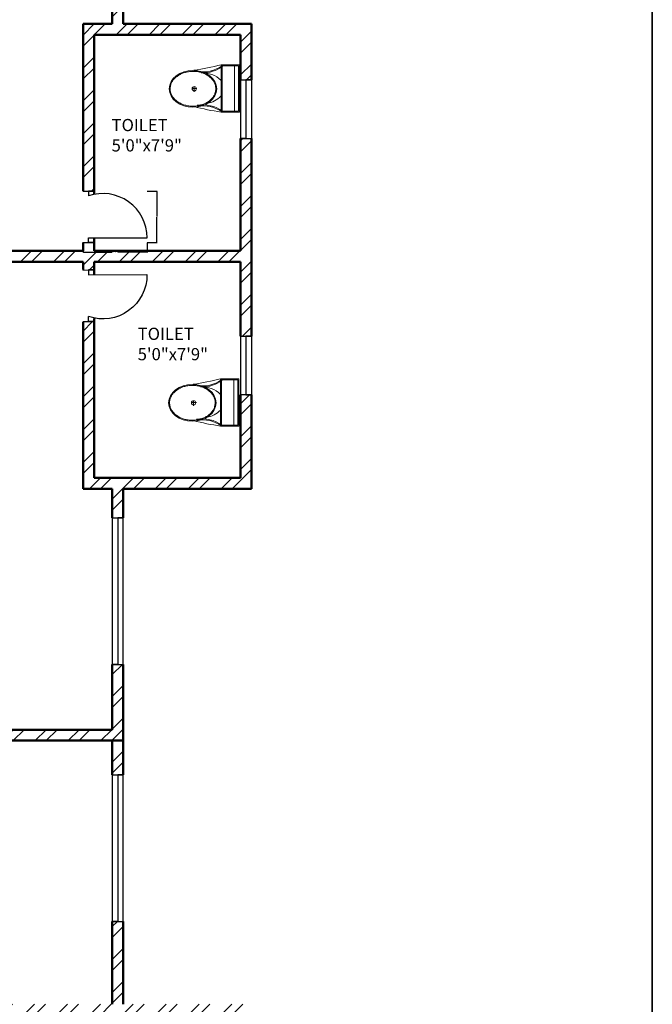
# Model space of a CAD drawing. Units: inches. Extents: x 963 to 2075, y 289 to 2657.
# Tile 58 of 98: x 1815 to 2075, y 1714 to 2117. Entities that reach past the tile are written whole.
import ezdxf

# ---------------------------------------------------------------- set-up
doc = ezdxf.new("R2010")
doc.units = ezdxf.units.IN
for name, color, linetype, lineweight in [('A-ANNO-DIMS', 2, 'Continuous', 18), ('A-ANNO-TTLB', 7, 'Continuous', 35), ('A-AREA-IDEN', 7, 'Continuous', 18), ('A-DOOR', 4, 'Continuous', 25), ('A-FLOR-FIXT', 9, 'Continuous', 18), ('A-GLAZ', 3, 'Continuous', 25), ('A-WALL', 7, 'Continuous', 50), ('A-WALL-PATT', 8, 'Continuous', 13)]:
    doc.layers.add(name, color=color, linetype=linetype, lineweight=lineweight)
doc.styles.get("Standard").update_dxf_attribs({"font": 'arial.ttf'})
doc.dimstyles.get("Standard").update_dxf_attribs({"dimtxt": 0.18, "dimasz": 0.18, "dimexe": 0.18, "dimexo": 0.0625, "dimgap": 0.09, "dimtad": 0, "dimtih": 1, "dimtoh": 1, "dimdec": 4, "dimzin": 0, "dimdsep": 46, "dimtxsty": 'Standard', "dimcen": 0.09, "dimadec": 0, "dimazin": 0, "dimtfac": 1, "dimtdec": 4, "dimtofl": 0, "dimtmove": 0, "dimatfit": 3, "dimfxl": 1, "dimtolj": 1, "dimtzin": 0, "dimarcsym": 0})

# ---------------------------------------------------------------- blocks, each defined once
blk = doc.blocks.new('A$C31115884')
for p, q in [((283, 498), (223, 498)), ((258, 466), (258, 523)), ((0, 200), (0, 0)), ((520, 200), (0, 200)), ((10, 190), (10, 10)), ((510, 190), (10, 190)), ((510, 10), (510, 190)), ((520, 0), (520, 200)), ((510, 54), (0, 54)), ((10, 10), (510, 10)), ((0, 0), (520, 0))]:
    blk.add_line(p, q)
blk.add_circle((256, 496), 23.6)
for centre, radius, start, end in [((2778, -205), 2807, 165.4549, 171.7133), ((-295, 403), 365, 324.2091, 9.3499), ((-295, 403), 375, 324.2091, 9.3499), ((806, 403), 365, 170.6501, 215.7909), ((3237, 905), 2807, 188.2867, 194.5451), ((384, 406), 293, 190.2774, 224.1564), ((139, 406), 293, 315.8436, 2.6563), ((806, 403), 375, 179.2036, 215.7909)]:
    blk.add_arc(centre, radius, start, end)
blk.add_ellipse((256, 510), major_axis=(0, -261), ratio=0.772727)
blk.add_open_spline([(256, 259), (263, 259), (270, 260), (288, 262), (299, 265), (320, 273), (330, 278), (350, 291), (360, 299), (378, 316), (386, 326), (402, 347), (409, 358), (421, 383), (427, 395), (436, 422), (440, 436), (445, 465), (447, 480), (448, 509), (448, 524), (445, 553), (443, 568), (436, 596), (432, 610), (422, 636), (416, 649), (402, 672), (395, 683), (379, 703), (370, 712), (351, 728), (341, 735), (321, 746), (310, 751), (289, 757), (278, 759), (256, 761), (245, 761), (223, 757), (212, 754), (191, 746), (181, 741), (161, 728), (151, 720), (133, 703), (125, 693), (110, 672), (103, 660), (90, 636), (85, 623), (76, 596), (72, 582), (67, 553), (66, 538), (64, 509), (65, 494), (68, 465), (70, 450), (77, 422), (81, 408), (91, 382), (97, 370), (111, 346), (118, 335), (135, 316), (144, 307), (162, 291), (172, 284), (193, 273), (203, 269), (225, 262), (236, 260), (250, 259), (253, 259), (256, 259)], degree=3, knots=[0, 0, 0, 0, 0.110105, 0.110105, 0.285049, 0.285049, 0.459994, 0.459994, 0.634938, 0.634938, 0.809882, 0.809882, 0.984827, 0.984827, 1.159771, 1.159771, 1.334715, 1.334715, 1.50966, 1.50966, 1.684604, 1.684604, 1.859549, 1.859549, 2.034493, 2.034493, 2.209437, 2.209437, 2.384382, 2.384382, 2.559326, 2.559326, 2.73427, 2.73427, 2.909215, 2.909215, 3.084159, 3.084159, 3.259103, 3.259103, 3.434048, 3.434048, 3.608992, 3.608992, 3.783936, 3.783936, 3.958881, 3.958881, 4.133825, 4.133825, 4.30877, 4.30877, 4.483714, 4.483714, 4.658658, 4.658658, 4.833603, 4.833603, 5.008547, 5.008547, 5.183491, 5.183491, 5.358436, 5.358436, 5.53338, 5.53338, 5.708324, 5.708324, 5.883269, 5.883269, 6.058213, 6.058213, 6.233158, 6.233158, 6.283185, 6.283185, 6.283185, 6.283185])
blk = doc.blocks.new('DOOR-2')
for p, q in [((0, 21.1), (4.5, 21.1)), ((4.5, 21.1), (2.25, 21.1)), ((2.25, 21.1), (2.25, 19.1)), ((0, 0), (4.5, 0)), ((2.25, 0), (2.25, 2)), ((2.25, 2), (26.25, 2)), ((4.5, 0), (2.25, 0))]:
    blk.add_line(p, q)
blk.add_arc((8.16, 2), 18.09, 0, 109.0656)
blk = doc.blocks.new('*D32')
at = {"layer": 'A-ANNO-DIMS', "color": 0, "lineweight": -2, "transparency": 16777216}
for p, q in [((1841.42, 2025.79), (1841.42, 2021.73)), ((1867.67, 2025.79), (1867.67, 2021.73)), ((1841.6, 2021.91), (1853.42, 2021.91)), ((1867.49, 2021.91), (1855.68, 2021.91))]:
    blk.add_line(p, q, dxfattribs=at)
at = {"layer": 'A-ANNO-DIMS', "color": 0, "transparency": 16777216}
for points in [[(1841.6, 2021.94), (1841.6, 2021.88), (1841.42, 2021.91)], [(1867.49, 2021.94), (1867.49, 2021.88), (1867.67, 2021.91)]]:
    blk.add_solid(points, dxfattribs=at)
at = {"layer": 'Defpoints', "color": 0, "transparency": 16777216}
for p in [(1841.42, 2025.85), (1867.67, 2025.85), (1867.67, 2021.91)]:
    blk.add_point(p, dxfattribs=at)
at = {"layer": 'A-ANNO-DIMS', "color": 0, "transparency": 16777216, "insert": (1854.55, 2021.91), "char_height": 0.18, "attachment_point": 5}
blk.add_mtext('\\A1;DOOR D2 26 TYP.', dxfattribs=at)
blk = doc.blocks.new('*D33')
at = {"layer": 'A-ANNO-DIMS', "color": 0, "lineweight": -2, "transparency": 16777216}
for p, q in [((1867.73, 2046.95), (1871.79, 2046.95)), ((1871.61, 2046.77), (1871.61, 2036.58)), ((1871.61, 2026.03), (1871.61, 2036.22)), ((1867.73, 2025.85), (1871.79, 2025.85))]:
    blk.add_line(p, q, dxfattribs=at)
at = {"layer": 'A-ANNO-DIMS', "color": 0, "transparency": 16777216}
for points in [[(1871.58, 2046.77), (1871.64, 2046.77), (1871.61, 2046.95)], [(1871.58, 2026.03), (1871.64, 2026.03), (1871.61, 2025.85)]]:
    blk.add_solid(points, dxfattribs=at)
at = {"layer": 'Defpoints', "color": 0, "transparency": 16777216}
for p in [(1867.67, 2046.95), (1871.61, 2046.95), (1867.67, 2025.85)]:
    blk.add_point(p, dxfattribs=at)
at = {"layer": 'A-ANNO-DIMS', "color": 0, "transparency": 16777216, "insert": (1871.61, 2036.4), "char_height": 0.18, "attachment_point": 5}
blk.add_mtext('\\A1;21 TYP.', dxfattribs=at)

msp = doc.modelspace()

# ---------------------------------------------------------------- hatches: boundary and pattern name
at = {"layer": 'A-WALL-PATT'}
h = msp.add_hatch(dxfattribs=at)
h.set_pattern_fill('ANSI32', color=256)
h.paths.add_polyline_path([(1296.92, 2558.32), (1203.92, 2558.32), (1203.92, 2493.82), (1191.53, 2493.82), (1191.53, 2489.32), (1211.06, 2489.32), (1211.06, 2492.02), (1211.06, 2493.82), (1208.42, 2493.82), (1208.42, 2553.82), (1292.42, 2553.82), (1292.42, 2538.86), (1296.92, 2538.86)])
h.paths.add_polyline_path([(1442.42, 2558.32), (1349.42, 2558.32), (1349.42, 2538.94), (1353.92, 2538.94), (1353.92, 2553.82), (1437.92, 2553.82), (1437.92, 2493.82), (1434.54, 2493.82), (1434.54, 2489.32), (1448.31, 2489.32), (1448.31, 2491.57), (1448.31, 2493.82), (1442.42, 2493.82)])
h.paths.add_polyline_path([(1415.55, 2491.57), (1415.55, 2493.82), (1340.94, 2493.82), (1340.94, 2489.32), (1371.92, 2489.32), (1371.92, 2378.32), (1367.6, 2378.32), (1367.6, 2373.82), (1371.92, 2373.82), (1371.92, 2355.19), (1376.42, 2355.19), (1376.42, 2489.32), (1415.55, 2489.32)])
h.paths.add_polyline_path([(1304.94, 2491.57), (1304.94, 2493.82), (1296.92, 2493.82), (1296.92, 2514.86), (1292.42, 2514.86), (1292.42, 2493.82), (1232.81, 2493.82), (1232.81, 2489.32), (1256.42, 2489.32), (1256.42, 2327.32), (1253.71, 2327.32), (1253.71, 2322.82), (1328.42, 2322.82), (1328.42, 2331.15), (1323.92, 2331.15), (1323.92, 2327.32), (1260.92, 2327.32), (1260.92, 2373.82), (1323.92, 2373.82), (1323.92, 2357.81), (1328.42, 2357.81), (1328.42, 2373.82), (1346.01, 2373.82), (1346.01, 2376.07), (1346.01, 2378.32), (1260.92, 2378.32), (1260.92, 2489.32), (1304.94, 2489.32)])
h.paths.add_polyline_path([(1226.65, 2327.32), (1124.42, 2327.32), (1124.42, 2347.45), (1119.92, 2347.45), (1119.92, 2322.82), (1163.42, 2322.82), (1163.42, 2305.43), (1165.67, 2305.43), (1167.92, 2305.43), (1167.92, 2322.82), (1226.65, 2322.82), (1226.65, 2325.07)])
h.paths.add_polyline_path([(1095.92, 2489.32), (1124.42, 2489.32), (1131.53, 2489.32), (1131.53, 2491.57), (1131.53, 2493.82), (1119.92, 2493.82), (1091.42, 2493.82), (1091.42, 2417.32), (1095.92, 2417.32), (1119.92, 2417.32), (1119.92, 2407.45), (1124.42, 2407.45), (1124.42, 2421.82), (1095.92, 2421.82)])
h.paths.add_polyline_path([(1512.92, 2558.32), (1508.42, 2558.32), (1508.42, 2493.82), (1503.4, 2493.82), (1503.4, 2489.32), (1508.42, 2489.32), (1508.42, 2327.32), (1376.42, 2327.32), (1376.42, 2330.27), (1371.92, 2330.27), (1371.92, 2298.74), (1376.42, 2298.74), (1376.42, 2322.82), (1508.42, 2322.82), (1508.42, 2165.32), (1504.26, 2165.32), (1504.26, 2160.82), (1508.42, 2160.82), (1508.42, 2108.32), (1512.92, 2108.32), (1512.92, 2160.82), (1516.18, 2160.82), (1516.18, 2163.07), (1516.18, 2165.32), (1512.92, 2165.32), (1512.92, 2322.82), (1644.92, 2322.82), (1644.92, 2298.74), (1649.42, 2298.74), (1649.42, 2322.82), (1649.42, 2330.94), (1647.17, 2330.94), (1644.92, 2330.94), (1644.92, 2327.32), (1512.92, 2327.32), (1512.92, 2489.32), (1516.76, 2489.32), (1516.76, 2491.57), (1516.76, 2493.82), (1512.92, 2493.82)])
h.paths.add_polyline_path([(1671.92, 2558.32), (1578.92, 2558.32), (1578.92, 2493.82), (1573.53, 2493.82), (1573.53, 2489.32), (1586.54, 2489.32), (1586.54, 2491.57), (1586.54, 2493.82), (1583.42, 2493.82), (1583.42, 2553.82), (1667.42, 2553.82), (1667.42, 2541.11), (1671.92, 2541.11)])
h.paths.add_polyline_path([(1681.26, 2493.82), (1671.92, 2493.82), (1671.92, 2517.11), (1667.42, 2517.11), (1667.42, 2493.82), (1610.22, 2493.82), (1610.22, 2489.32), (1644.92, 2489.32), (1644.92, 2357.87), (1649.42, 2357.87), (1649.42, 2373.82), (1652.2, 2373.82), (1652.2, 2375.83), (1652.2, 2378.32), (1649.42, 2378.32), (1649.42, 2489.32), (1681.26, 2489.32), (1681.26, 2491.57)])
h.paths.add_polyline_path([(1821.92, 2558.32), (1728.92, 2558.32), (1728.92, 2541), (1733.42, 2541), (1733.42, 2553.82), (1817.42, 2553.82), (1817.42, 2493.82), (1813.51, 2493.82), (1813.51, 2489.32), (1830.08, 2489.32), (1830.08, 2491.57), (1830.08, 2493.82), (1821.92, 2493.82)])
h.paths.add_polyline_path([(1794.24, 2493.82), (1717.26, 2493.82), (1717.26, 2489.32), (1760.42, 2489.32), (1760.42, 2378.32), (1674.4, 2378.32), (1674.4, 2373.82), (1692.92, 2373.82), (1692.92, 2356.95), (1697.42, 2356.95), (1697.42, 2373.82), (1760.42, 2373.82), (1760.42, 2327.32), (1697.42, 2327.32), (1697.42, 2333.34), (1692.92, 2333.34), (1692.92, 2322.82), (1768.04, 2322.82), (1768.04, 2325.07), (1768.04, 2327.32), (1764.92, 2327.32), (1764.92, 2489.32), (1794.24, 2489.32)])
h.paths.add_polyline_path([(1733.42, 2517), (1728.92, 2517), (1728.92, 2493.82), (1733.42, 2493.82)], flags=17)
h.paths.add_polyline_path([(1929.92, 2493.82), (1890.08, 2493.82), (1890.08, 2489.32), (1896.92, 2489.32), (1925.42, 2489.32), (1925.42, 2421.82), (1896.92, 2421.82), (1896.92, 2408.32), (1901.42, 2408.32), (1901.42, 2417.32), (1925.42, 2417.32), (1929.92, 2417.32)])
h.paths.add_polyline_path([(1901.42, 2348.32), (1896.92, 2348.32), (1896.92, 2327.32), (1800.42, 2327.32), (1800.42, 2322.82), (1853.42, 2322.82), (1853.42, 2309.45), (1857.92, 2309.45), (1857.92, 2322.82), (1901.42, 2322.82)])
h.paths.add_polyline_path([(1857.92, 2249.45), (1853.42, 2249.45), (1853.42, 2214.82), (1686.31, 2214.82), (1686.31, 2210.32), (1853.42, 2210.32), (1853.42, 2202.13), (1857.92, 2202.13), (1857.92, 2210.32)])
h.paths.add_polyline_path([(1857.92, 2142.13), (1853.42, 2142.13), (1853.42, 2115.42), (1841.42, 2115.42), (1841.42, 2088.53), (1841.42, 2046.95), (1845.92, 2046.95), (1845.92, 2110.92), (1905.92, 2110.92), (1905.92, 2092.52), (1910.42, 2092.52), (1910.42, 2115.42), (1857.92, 2115.42)])
h.paths.add_polyline_path([(1532.44, 1482.34), (1573.46, 1482.34), (1573.46, 1501), (1532.44, 1501)], flags=9)
h.paths.add_polyline_path([(1438.66, 1486.3), (1479.68, 1486.3), (1479.68, 1504.96), (1438.66, 1504.96)], flags=9)
h.paths.add_polyline_path([(1411.22, 1365.31), (1659.14, 1365.31), (1659.14, 1402.4), (1411.22, 1402.4)], flags=9)
h.paths.add_polyline_path([(1185.67, 2296.3), (1248.16, 2296.3), (1248.16, 2314.95), (1185.67, 2314.95)], flags=9)
h.paths.add_polyline_path([(1177.31, 2187.35), (1216.15, 2187.35), (1216.15, 2206.01), (1177.31, 2206.01)], flags=9)
h.paths.add_polyline_path([(1295.1, 1602.08), (1328.26, 1602.08), (1328.26, 1620.74), (1295.1, 1620.74)], flags=9)
h.paths.add_polyline_path([(1525.13, 2005.99), (1558.39, 2005.99), (1558.39, 2024.65), (1525.13, 2024.65)], flags=9)
h.paths.add_polyline_path([(1459.61, 1977.13), (1472.19, 1977.13), (1472.19, 1987.43), (1459.61, 1987.43)], flags=9)
h.paths.add_polyline_path([(1467.81, 2053.68), (1480.02, 2053.68), (1480.02, 2063.98), (1467.81, 2063.98)], flags=9)
h.paths.add_polyline_path([(1555.18, 2119.02), (1584.56, 2119.02), (1584.56, 2137.68), (1555.18, 2137.68)], flags=25)
h.paths.add_polyline_path([(1405.39, 2115.29), (1444.48, 2115.29), (1444.48, 2133.95), (1405.39, 2133.95)], flags=25)
h.paths.add_polyline_path([(1698.48, 2004.26), (1727.69, 2004.26), (1727.69, 2022.92), (1698.48, 2022.92)], flags=9)
h.paths.add_polyline_path([(1612.16, 1972.86), (1629.02, 1972.86), (1629.02, 1983.16), (1612.16, 1983.16)], flags=9)
h.paths.add_polyline_path([(1608.29, 2060.04), (1625.15, 2060.04), (1625.15, 2070.34), (1608.29, 2070.34)], flags=9)
h.paths.add_polyline_path([(1527.95, 1684.4), (1566.79, 1684.4), (1566.79, 1703.06), (1527.95, 1703.06)], flags=9)
h.paths.add_polyline_path([(1422.79, 1683.59), (1461.63, 1683.59), (1461.63, 1702.25), (1422.79, 1702.25)], flags=9)
h.paths.add_polyline_path([(1531.26, 1732.46), (1574.01, 1732.46), (1574.01, 1751.12), (1531.26, 1751.12)], flags=9)
h.paths.add_polyline_path([(1402.87, 1732.85), (1439.8, 1732.85), (1439.8, 1751.5), (1402.87, 1751.5)], flags=9)
h.paths.add_polyline_path([(1243.12, 1923.13), (1281.96, 1923.13), (1281.96, 1941.79), (1243.12, 1941.79)], flags=9)
h.paths.add_polyline_path([(1181.75, 1792.27), (1244.24, 1792.27), (1244.24, 1810.93), (1181.75, 1810.93)], flags=9)
h.paths.add_polyline_path([(1265.82, 1670.3), (1316.07, 1670.3), (1316.07, 1688.96), (1265.82, 1688.96)], flags=9)
h.paths.add_polyline_path([(1140.26, 1676.05), (1179.1, 1676.05), (1179.1, 1694.71), (1140.26, 1694.71)], flags=9)
h.paths.add_polyline_path([(1107.49, 1490.89), (1143.37, 1490.89), (1143.37, 1509.55), (1107.49, 1509.55)], flags=9)
h.paths.add_polyline_path([(1217.58, 1483.9), (1246.74, 1483.9), (1246.74, 1502.56), (1217.58, 1502.56)], flags=9)
h.paths.add_polyline_path([(1389.21, 1486.92), (1418.37, 1486.92), (1418.37, 1505.58), (1389.21, 1505.58)], flags=9)
h.paths.add_polyline_path([(1672.21, 1602.08), (1705.37, 1602.08), (1705.37, 1620.74), (1672.21, 1620.74)], flags=9)
h.paths.add_polyline_path([(1752.08, 1522.64), (1781.24, 1522.64), (1781.24, 1541.3), (1752.08, 1541.3)], flags=9)
h.paths.add_polyline_path([(1848.27, 1491.26), (1884.16, 1491.26), (1884.16, 1509.92), (1848.27, 1509.92)], flags=9)
h.paths.add_polyline_path([(1822.47, 1685.62), (1861.31, 1685.62), (1861.31, 1704.28), (1822.47, 1704.28)], flags=9)
h.paths.add_polyline_path([(1713.19, 1672.23), (1763.44, 1672.23), (1763.44, 1690.89), (1713.19, 1690.89)], flags=9)
h.paths.add_polyline_path([(1736.62, 1790.58), (1799.11, 1790.58), (1799.11, 1809.24), (1736.62, 1809.24)], flags=9)
h.paths.add_polyline_path([(1691.49, 1916.36), (1730.33, 1916.36), (1730.33, 1935.01), (1691.49, 1935.01)], flags=9)
h.paths.add_polyline_path([(1764.87, 1973.92), (1794.31, 1973.92), (1794.31, 1992.58), (1764.87, 1992.58)], flags=9)
h.paths.add_polyline_path([(1767.85, 2034.02), (1797.29, 2034.02), (1797.29, 2052.67), (1767.85, 2052.67)], flags=9)
h.paths.add_polyline_path([(1851.59, 2060.33), (1880.75, 2060.33), (1880.75, 2078.99), (1851.59, 2078.99)], flags=25)
h.paths.add_polyline_path([(1688.49, 2086.87), (1727.33, 2086.87), (1727.33, 2105.53), (1688.49, 2105.53)], flags=9)
h.paths.add_polyline_path([(1537.74, 2293.58), (1580.49, 2293.58), (1580.49, 2312.24), (1537.74, 2312.24)], flags=25)
h.paths.add_polyline_path([(1425.59, 2296.11), (1468.34, 2296.11), (1468.34, 2314.77), (1425.59, 2314.77)], flags=25)
h.paths.add_polyline_path([(1278.52, 2004.18), (1307.72, 2004.18), (1307.72, 2022.84), (1278.52, 2022.84)], flags=9)
h.paths.add_polyline_path([(1193.28, 1973.63), (1222.72, 1973.63), (1222.72, 1992.29), (1193.28, 1992.29)], flags=9)
h.paths.add_polyline_path([(1192.41, 2040.58), (1221.84, 2040.58), (1221.84, 2059.23), (1192.41, 2059.23)], flags=9)
h.paths.add_polyline_path([(1130.6, 1951.39), (1159.76, 1951.39), (1159.76, 1970.05), (1130.6, 1970.05)], flags=9)
h.paths.add_polyline_path([(1132.83, 2052.49), (1161.98, 2052.49), (1161.98, 2071.15), (1132.83, 2071.15)], flags=9)
h.paths.add_polyline_path([(1265.13, 2334.62), (1315.38, 2334.62), (1315.38, 2353.28), (1265.13, 2353.28)], flags=25)
h.paths.add_polyline_path([(1136.74, 2330.79), (1175.58, 2330.79), (1175.58, 2349.44), (1136.74, 2349.44)], flags=9)
h.paths.add_polyline_path([(1287.42, 2417.2), (1320.58, 2417.2), (1320.58, 2435.86), (1287.42, 2435.86)], flags=25)
h.paths.add_polyline_path([(1430.99, 2329.16), (1469.83, 2329.16), (1469.83, 2347.82), (1430.99, 2347.82)], flags=25)
h.paths.add_polyline_path([(1525.42, 2329.21), (1564.26, 2329.21), (1564.26, 2347.87), (1525.42, 2347.87)], flags=25)
h.paths.add_polyline_path([(1684.52, 2382.8), (1717.68, 2382.8), (1717.68, 2401.46), (1684.52, 2401.46)], flags=25)
h.paths.add_polyline_path([(1704.81, 2340.29), (1755.05, 2340.29), (1755.05, 2358.95), (1704.81, 2358.95)], flags=25)
h.paths.add_polyline_path([(1694.11, 2287.76), (1756.6, 2287.76), (1756.6, 2306.41), (1694.11, 2306.41)], flags=9)
h.paths.add_polyline_path([(1815.78, 2329.86), (1854.62, 2329.86), (1854.62, 2348.52), (1815.78, 2348.52)], flags=9)
h.paths.add_polyline_path([(1842.87, 2514.26), (1878.76, 2514.26), (1878.76, 2532.91), (1842.87, 2532.91)], flags=9)
h.paths.add_polyline_path([(1769.51, 2531.45), (1798.67, 2531.45), (1798.67, 2550.1), (1769.51, 2550.1)], flags=25)
h.paths.add_polyline_path([(1594.77, 2518.47), (1623.93, 2518.47), (1623.93, 2537.13), (1594.77, 2537.13)], flags=25)
h.paths.add_polyline_path([(1520.72, 2516.18), (1556.61, 2516.18), (1556.61, 2534.84), (1520.72, 2534.84)], flags=25)
h.paths.add_polyline_path([(1464.46, 2516.69), (1500.34, 2516.69), (1500.34, 2535.35), (1464.46, 2535.35)], flags=25)
h.paths.add_polyline_path([(1365.7, 2528.97), (1394.85, 2528.97), (1394.85, 2547.63), (1365.7, 2547.63)], flags=25)
h.paths.add_polyline_path([(1222.84, 2516.23), (1252, 2516.23), (1252, 2534.89), (1222.84, 2534.89)], flags=25)
h.paths.add_polyline_path([(1104.55, 2509.6), (1140.43, 2509.6), (1140.43, 2528.26), (1104.55, 2528.26)], flags=9)
h = msp.add_hatch(dxfattribs=at)
h.set_pattern_fill('ANSI32', color=256)
h.paths.add_polyline_path([(1335.97, 2212.57), (1335.97, 2214.82), (1167.92, 2214.82), (1167.92, 2245.43), (1163.42, 2245.43), (1163.42, 2210.32), (1163.42, 2194.81), (1167.92, 2194.81), (1167.92, 2210.32), (1335.97, 2210.32)])
h.paths.add_polyline_path([(1532.44, 1482.34), (1573.46, 1482.34), (1573.46, 1501), (1532.44, 1501)], flags=9)
h.paths.add_polyline_path([(1438.66, 1486.3), (1479.68, 1486.3), (1479.68, 1504.96), (1438.66, 1504.96)], flags=9)
h.paths.add_polyline_path([(1411.22, 1365.31), (1659.14, 1365.31), (1659.14, 1402.4), (1411.22, 1402.4)], flags=9)
h.paths.add_polyline_path([(1185.67, 2296.3), (1248.16, 2296.3), (1248.16, 2314.95), (1185.67, 2314.95)], flags=9)
h.paths.add_polyline_path([(1177.31, 2187.35), (1216.15, 2187.35), (1216.15, 2206.01), (1177.31, 2206.01)], flags=9)
h.paths.add_polyline_path([(1295.1, 1602.08), (1328.26, 1602.08), (1328.26, 1620.74), (1295.1, 1620.74)], flags=9)
h.paths.add_polyline_path([(1525.13, 2005.99), (1558.39, 2005.99), (1558.39, 2024.65), (1525.13, 2024.65)], flags=9)
h.paths.add_polyline_path([(1459.61, 1977.13), (1472.19, 1977.13), (1472.19, 1987.43), (1459.61, 1987.43)], flags=9)
h.paths.add_polyline_path([(1467.81, 2053.68), (1480.02, 2053.68), (1480.02, 2063.98), (1467.81, 2063.98)], flags=9)
h.paths.add_polyline_path([(1555.18, 2119.02), (1584.56, 2119.02), (1584.56, 2137.68), (1555.18, 2137.68)], flags=9)
h.paths.add_polyline_path([(1405.39, 2115.29), (1444.48, 2115.29), (1444.48, 2133.95), (1405.39, 2133.95)], flags=9)
h.paths.add_polyline_path([(1698.48, 2004.26), (1727.69, 2004.26), (1727.69, 2022.92), (1698.48, 2022.92)], flags=9)
h.paths.add_polyline_path([(1612.16, 1972.86), (1629.02, 1972.86), (1629.02, 1983.16), (1612.16, 1983.16)], flags=9)
h.paths.add_polyline_path([(1608.29, 2060.04), (1625.15, 2060.04), (1625.15, 2070.34), (1608.29, 2070.34)], flags=9)
h.paths.add_polyline_path([(1527.95, 1684.4), (1566.79, 1684.4), (1566.79, 1703.06), (1527.95, 1703.06)], flags=9)
h.paths.add_polyline_path([(1422.79, 1683.59), (1461.63, 1683.59), (1461.63, 1702.25), (1422.79, 1702.25)], flags=9)
h.paths.add_polyline_path([(1531.26, 1732.46), (1574.01, 1732.46), (1574.01, 1751.12), (1531.26, 1751.12)], flags=9)
h.paths.add_polyline_path([(1402.87, 1732.85), (1439.8, 1732.85), (1439.8, 1751.5), (1402.87, 1751.5)], flags=9)
h.paths.add_polyline_path([(1243.12, 1923.13), (1281.96, 1923.13), (1281.96, 1941.79), (1243.12, 1941.79)], flags=9)
h.paths.add_polyline_path([(1181.75, 1792.27), (1244.24, 1792.27), (1244.24, 1810.93), (1181.75, 1810.93)], flags=9)
h.paths.add_polyline_path([(1265.82, 1670.3), (1316.07, 1670.3), (1316.07, 1688.96), (1265.82, 1688.96)], flags=9)
h.paths.add_polyline_path([(1140.26, 1676.05), (1179.1, 1676.05), (1179.1, 1694.71), (1140.26, 1694.71)], flags=9)
h.paths.add_polyline_path([(1107.49, 1490.89), (1143.37, 1490.89), (1143.37, 1509.55), (1107.49, 1509.55)], flags=9)
h.paths.add_polyline_path([(1217.58, 1483.9), (1246.74, 1483.9), (1246.74, 1502.56), (1217.58, 1502.56)], flags=9)
h.paths.add_polyline_path([(1389.21, 1486.92), (1418.37, 1486.92), (1418.37, 1505.58), (1389.21, 1505.58)], flags=9)
h.paths.add_polyline_path([(1672.21, 1602.08), (1705.37, 1602.08), (1705.37, 1620.74), (1672.21, 1620.74)], flags=9)
h.paths.add_polyline_path([(1752.08, 1522.64), (1781.24, 1522.64), (1781.24, 1541.3), (1752.08, 1541.3)], flags=9)
h.paths.add_polyline_path([(1848.27, 1491.26), (1884.16, 1491.26), (1884.16, 1509.92), (1848.27, 1509.92)], flags=9)
h.paths.add_polyline_path([(1822.47, 1685.62), (1861.31, 1685.62), (1861.31, 1704.28), (1822.47, 1704.28)], flags=9)
h.paths.add_polyline_path([(1713.19, 1672.23), (1763.44, 1672.23), (1763.44, 1690.89), (1713.19, 1690.89)], flags=9)
h.paths.add_polyline_path([(1736.62, 1790.58), (1799.11, 1790.58), (1799.11, 1809.24), (1736.62, 1809.24)], flags=9)
h.paths.add_polyline_path([(1691.49, 1916.36), (1730.33, 1916.36), (1730.33, 1935.01), (1691.49, 1935.01)], flags=9)
h.paths.add_polyline_path([(1764.87, 1973.92), (1794.31, 1973.92), (1794.31, 1992.58), (1764.87, 1992.58)], flags=9)
h.paths.add_polyline_path([(1767.85, 2034.02), (1797.29, 2034.02), (1797.29, 2052.67), (1767.85, 2052.67)], flags=9)
h.paths.add_polyline_path([(1851.59, 2060.33), (1880.75, 2060.33), (1880.75, 2078.99), (1851.59, 2078.99)], flags=9)
h.paths.add_polyline_path([(1688.49, 2086.87), (1727.33, 2086.87), (1727.33, 2105.53), (1688.49, 2105.53)], flags=9)
h.paths.add_polyline_path([(1537.74, 2293.58), (1580.49, 2293.58), (1580.49, 2312.24), (1537.74, 2312.24)], flags=9)
h.paths.add_polyline_path([(1425.59, 2296.11), (1468.34, 2296.11), (1468.34, 2314.77), (1425.59, 2314.77)], flags=9)
h.paths.add_polyline_path([(1278.52, 2004.18), (1307.72, 2004.18), (1307.72, 2022.84), (1278.52, 2022.84)], flags=9)
h.paths.add_polyline_path([(1193.28, 1973.63), (1222.72, 1973.63), (1222.72, 1992.29), (1193.28, 1992.29)], flags=9)
h.paths.add_polyline_path([(1192.41, 2040.58), (1221.84, 2040.58), (1221.84, 2059.23), (1192.41, 2059.23)], flags=9)
h.paths.add_polyline_path([(1130.6, 1951.39), (1159.76, 1951.39), (1159.76, 1970.05), (1130.6, 1970.05)], flags=9)
h.paths.add_polyline_path([(1132.83, 2052.49), (1161.98, 2052.49), (1161.98, 2071.15), (1132.83, 2071.15)], flags=9)
h.paths.add_polyline_path([(1265.13, 2334.62), (1315.38, 2334.62), (1315.38, 2353.28), (1265.13, 2353.28)], flags=9)
h.paths.add_polyline_path([(1136.74, 2330.79), (1175.58, 2330.79), (1175.58, 2349.44), (1136.74, 2349.44)], flags=9)
h.paths.add_polyline_path([(1287.42, 2417.2), (1320.58, 2417.2), (1320.58, 2435.86), (1287.42, 2435.86)], flags=9)
h.paths.add_polyline_path([(1430.99, 2329.16), (1469.83, 2329.16), (1469.83, 2347.82), (1430.99, 2347.82)], flags=9)
h.paths.add_polyline_path([(1525.42, 2329.21), (1564.26, 2329.21), (1564.26, 2347.87), (1525.42, 2347.87)], flags=9)
h.paths.add_polyline_path([(1684.52, 2382.8), (1717.68, 2382.8), (1717.68, 2401.46), (1684.52, 2401.46)], flags=9)
h.paths.add_polyline_path([(1704.81, 2340.29), (1755.05, 2340.29), (1755.05, 2358.95), (1704.81, 2358.95)], flags=9)
h.paths.add_polyline_path([(1694.11, 2287.76), (1756.6, 2287.76), (1756.6, 2306.41), (1694.11, 2306.41)], flags=9)
h.paths.add_polyline_path([(1815.78, 2329.86), (1854.62, 2329.86), (1854.62, 2348.52), (1815.78, 2348.52)], flags=9)
h.paths.add_polyline_path([(1842.87, 2514.26), (1878.76, 2514.26), (1878.76, 2532.91), (1842.87, 2532.91)], flags=9)
h.paths.add_polyline_path([(1769.51, 2531.45), (1798.67, 2531.45), (1798.67, 2550.1), (1769.51, 2550.1)], flags=9)
h.paths.add_polyline_path([(1594.77, 2518.47), (1623.93, 2518.47), (1623.93, 2537.13), (1594.77, 2537.13)], flags=9)
h.paths.add_polyline_path([(1520.72, 2516.18), (1556.61, 2516.18), (1556.61, 2534.84), (1520.72, 2534.84)], flags=9)
h.paths.add_polyline_path([(1464.46, 2516.69), (1500.34, 2516.69), (1500.34, 2535.35), (1464.46, 2535.35)], flags=9)
h.paths.add_polyline_path([(1365.7, 2528.97), (1394.85, 2528.97), (1394.85, 2547.63), (1365.7, 2547.63)], flags=9)
h.paths.add_polyline_path([(1222.84, 2516.23), (1252, 2516.23), (1252, 2534.89), (1222.84, 2534.89)], flags=9)
h.paths.add_polyline_path([(1104.55, 2509.6), (1140.43, 2509.6), (1140.43, 2528.26), (1104.55, 2528.26)], flags=9)
h = msp.add_hatch(dxfattribs=at)
h.set_pattern_fill('ANSI32', color=256)
h.paths.add_polyline_path([(1473.61, 2163.07), (1473.61, 2165.32), (1376.42, 2165.32), (1376.42, 2227.98), (1371.92, 2227.98), (1371.92, 2214.82), (1368.41, 2214.82), (1368.41, 2210.32), (1371.92, 2210.32), (1371.92, 2160.82), (1395.92, 2160.82), (1395.92, 2090.32), (1217.34, 2090.32), (1217.34, 2085.82), (1395.92, 2085.82), (1458.92, 2085.82), (1458.92, 2108.32), (1454.42, 2108.32), (1454.42, 2090.32), (1400.42, 2090.32), (1400.42, 2160.82), (1473.61, 2160.82)])
h.paths.add_polyline_path([(1649.42, 2210.32), (1653.23, 2210.32), (1653.23, 2214.82), (1649.42, 2214.82), (1649.42, 2227.98), (1644.92, 2227.98), (1644.92, 2165.32), (1550.1, 2165.32), (1550.1, 2160.82), (1620.92, 2160.82), (1620.92, 2112.82), (1555.45, 2112.82), (1555.45, 2108.32), (1584.33, 2108.32), (1584.33, 2084.92), (1588.83, 2084.92), (1588.83, 2108.32), (1625.42, 2108.32), (1667.95, 2108.32), (1667.95, 2022.67), (1588.83, 2022.67), (1588.83, 2047.41), (1584.33, 2047.41), (1584.33, 1996), (1588.83, 1996), (1588.83, 2018.32), (1667.95, 2018.17), (1667.95, 1928.32), (1625.42, 1928.32), (1625.42, 1923.82), (1672.45, 1923.82), (1672.45, 1928.32), (1672.45, 1946.66), (1785.45, 1946.66), (1785.45, 1951.16), (1743.03, 1951.16), (1743.03, 2017.92), (1841.42, 2017.92), (1841.42, 2014.77), (1845.92, 2014.77), (1845.92, 2017.92), (1905.92, 2017.92), (1905.92, 1987.51), (1910.42, 1987.51), (1910.42, 2022.42), (1910.42, 2068.52), (1905.92, 2068.52), (1905.92, 2022.42), (1845.92, 2022.42), (1845.92, 2025.85), (1843.67, 2025.85), (1841.42, 2025.85), (1841.42, 2022.42), (1743.03, 2022.42), (1743.03, 2084.03), (1768.45, 2084.03), (1785.45, 2084.03), (1785.45, 2088.53), (1672.45, 2088.53), (1672.45, 2112.82), (1667.95, 2112.82), (1625.42, 2112.82), (1625.42, 2160.82), (1649.42, 2160.82)])
h.paths.add_polyline_path([(1672.45, 2084.03), (1738.53, 2084.03), (1738.53, 1951.16), (1672.45, 1951.16)], flags=16)
h.paths.add_polyline_path([(1672.45, 2084.03), (1738.53, 2084.03), (1705.49, 2017.6)], flags=0)
h.paths.add_polyline_path([(1262.77, 2085.82), (1258.27, 2085.82), (1258.27, 2023.28), (1184.42, 2023.28), (1184.42, 2018.78), (1258.27, 2018.78), (1258.27, 1950.82), (1262.77, 1950.82)])
h.paths.add_polyline_path([(1312.27, 2085.82), (1307.77, 2085.82), (1307.77, 1950.82), (1312.27, 1950.82)])
h.paths.add_polyline_path([(1458.92, 1950.82), (1395.92, 1950.82), (1216.57, 1950.82), (1216.57, 1946.32), (1346.42, 1946.32), (1395.92, 1946.32), (1395.92, 1875.82), (1371.92, 1875.82), (1371.92, 1826.32), (1368.93, 1826.32), (1368.93, 1821.82), (1371.92, 1821.82), (1371.92, 1813.62), (1376.42, 1813.62), (1376.42, 1871.32), (1474.5, 1871.32), (1474.5, 1873.57), (1474.5, 1875.82), (1400.42, 1875.82), (1400.42, 1946.32), (1454.42, 1946.32), (1454.42, 1928.32), (1458.92, 1928.32)])
h.paths.add_polyline_path([(1184.42, 2120.78), (1167.92, 2120.78), (1167.92, 2134.81), (1165.67, 2134.81), (1163.42, 2134.81), (1163.42, 2120.78), (1119.92, 2120.78), (1119.92, 2098.1), (1124.42, 2098.1), (1124.42, 2116.28), (1167.92, 2116.28), (1179.92, 2116.28), (1179.92, 2045.92), (1184.42, 2045.92), (1184.42, 2090.32), (1184.42, 2116.28)])
h.paths.add_polyline_path([(1124.42, 2018.78), (1179.92, 2018.78), (1179.92, 2016.29), (1184.42, 2016.29), (1184.42, 2023.28), (1184.42, 2026.59), (1182.17, 2026.59), (1179.92, 2026.59), (1179.92, 2023.28), (1124.42, 2023.28), (1124.42, 2074.1), (1119.92, 2074.1), (1119.92, 2018.78), (1119.92, 1979.63), (1124.42, 1979.63)])
h.paths.add_polyline_path([(1184.42, 1925.78), (1184.42, 1946.32), (1184.42, 1996.07), (1182.17, 1996.07), (1179.92, 1996.07), (1179.92, 1925.78), (1124.42, 1925.78), (1124.42, 1955.63), (1119.92, 1955.5), (1119.92, 1921.28), (1158.92, 1921.28), (1158.92, 1909.98), (1163.42, 1909.98), (1163.42, 1921.28), (1184.42, 1921.28)])
h.paths.add_polyline_path([(1341.45, 1826.32), (1163.42, 1826.32), (1163.42, 1849.98), (1158.92, 1849.98), (1158.92, 1821.82), (1158.92, 1804.03), (1163.42, 1804.03), (1163.42, 1821.82), (1341.45, 1821.82)])
h.paths.add_polyline_path([(1222.98, 1713.82), (1163.42, 1713.82), (1163.42, 1744.03), (1161.17, 1744.03), (1158.92, 1744.03), (1158.92, 1713.82), (1119.92, 1713.82), (1119.92, 1694.65), (1124.42, 1694.65), (1124.42, 1709.32), (1158.92, 1709.32), (1222.98, 1709.32)])
h.paths.add_polyline_path([(1328.42, 1713.82), (1252.04, 1713.82), (1252.04, 1711.57), (1252.04, 1709.32), (1256.42, 1709.32), (1256.42, 1547.32), (1232.94, 1547.32), (1232.94, 1545.07), (1232.94, 1542.82), (1292.42, 1542.82), (1292.42, 1527.63), (1296.92, 1527.63), (1296.92, 1542.82), (1299.46, 1542.82), (1299.46, 1547.32), (1260.92, 1547.32), (1260.92, 1658.32), (1343.66, 1658.32), (1343.66, 1660.57), (1343.66, 1662.82), (1328.42, 1662.82), (1328.42, 1676.59), (1327.4, 1676.59), (1323.92, 1676.59), (1323.92, 1662.82), (1260.92, 1662.82), (1260.92, 1709.32), (1323.92, 1709.32), (1323.92, 1699.85), (1328.42, 1699.85)])
h.paths.add_polyline_path([(1649.42, 1875.82), (1625.42, 1875.82), (1625.42, 1928.32), (1620.92, 1928.32), (1588.83, 1928.32), (1588.83, 1950.59), (1584.33, 1950.59), (1584.33, 1928.32), (1555.45, 1928.32), (1555.45, 1923.82), (1620.92, 1923.82), (1620.92, 1875.82), (1548.95, 1875.82), (1548.95, 1873.57), (1548.95, 1871.32), (1644.92, 1871.32), (1644.92, 1813.62), (1649.42, 1813.62), (1649.42, 1821.82), (1652.04, 1821.82), (1652.04, 1824.07), (1652.04, 1826.32), (1649.42, 1826.32)])
h.paths.add_polyline_path([(1512.92, 1871.32), (1516.48, 1871.32), (1516.48, 1875.82), (1512.92, 1875.82), (1512.92, 1923.82), (1512.92, 1928.32), (1512.92, 1930.83), (1508.42, 1930.83), (1508.42, 1875.82), (1504.41, 1875.82), (1504.41, 1871.32), (1508.42, 1871.32), (1508.42, 1713.82), (1376.42, 1713.82), (1376.42, 1743.32), (1371.92, 1743.32), (1371.92, 1709.32), (1371.92, 1706.01), (1376.42, 1706.01), (1376.42, 1709.32), (1508.42, 1709.32), (1508.42, 1547.32), (1501.87, 1547.32), (1501.87, 1542.82), (1508.42, 1542.82), (1508.42, 1482.82), (1508.42, 1436.32), (1512.92, 1436.32), (1512.92, 1542.82), (1519.32, 1542.82), (1519.32, 1545.07), (1519.32, 1547.32), (1512.92, 1547.32), (1512.92, 1709.32), (1644.92, 1709.32), (1644.92, 1707.55), (1649.42, 1707.55), (1649.42, 1709.32), (1649.42, 1743.32), (1644.92, 1743.32), (1644.92, 1713.82), (1512.92, 1713.82)])
h.paths.add_polyline_path([(1129.88, 1545.07), (1129.88, 1547.32), (1124.42, 1547.32), (1095.92, 1547.32), (1095.92, 1614.82), (1124.42, 1614.82), (1124.42, 1619.32), (1095.92, 1619.32), (1091.42, 1619.32), (1091.42, 1542.82), (1095.92, 1542.82), (1119.92, 1542.82), (1129.88, 1542.82)])
h.paths.add_polyline_path([(1208.42, 1542.82), (1211.74, 1542.82), (1211.74, 1547.32), (1198.85, 1547.32), (1198.85, 1542.82), (1203.92, 1542.82), (1203.92, 1478.32), (1208.42, 1478.32), (1296.92, 1478.32), (1296.92, 1503.63), (1292.42, 1503.63), (1292.42, 1482.82), (1208.42, 1482.82)])
h.paths.add_polyline_path([(1430.42, 1542.82), (1435.7, 1542.82), (1435.7, 1545.07), (1435.7, 1547.32), (1422.66, 1547.32), (1422.66, 1545.07), (1422.66, 1542.82), (1425.92, 1542.82), (1425.92, 1482.86), (1341.92, 1482.86), (1341.92, 1502.73), (1337.42, 1502.73), (1337.42, 1478.36), (1425.92, 1478.36), (1425.92, 1440.82), (1425.92, 1436.32), (1430.42, 1436.32)])
h.paths.add_polyline_path([(1698.48, 2004.26), (1727.69, 2004.26), (1727.69, 2022.92), (1698.48, 2022.92)], flags=8)
h = msp.add_hatch(dxfattribs=at)
h.set_pattern_fill('ANSI32', color=256)
h.paths.add_polyline_path([(1910.42, 1929.42), (1910.42, 1963.51), (1905.92, 1963.51), (1905.92, 1929.42), (1845.92, 1929.42), (1845.92, 1993.37), (1843.67, 1993.37), (1841.42, 1993.37), (1841.42, 1951.16), (1841.42, 1924.92), (1853.42, 1924.92), (1853.42, 1913.07), (1857.92, 1913.07), (1857.92, 1924.92), (1910.42, 1924.92)])
h.paths.add_polyline_path([(1857.92, 1853.07), (1853.42, 1853.07), (1853.42, 1826.32), (1841.42, 1826.32), (1674.48, 1826.32), (1674.48, 1821.82), (1853.42, 1821.82), (1857.92, 1821.82)])
h.paths.add_polyline_path([(1857.92, 1821.82), (1853.42, 1821.82), (1853.42, 1807.79), (1857.92, 1807.79)])
h.paths.add_polyline_path([(1857.92, 1747.79), (1853.42, 1747.79), (1853.42, 1713.82), (1809.34, 1713.82), (1809.34, 1709.32), (1905.92, 1709.32), (1905.92, 1688.32), (1910.42, 1688.32), (1910.42, 1713.82), (1857.92, 1713.82)])
h.paths.add_polyline_path([(1830.92, 1542.82), (1837.43, 1542.82), (1837.43, 1545.07), (1837.43, 1547.32), (1823.42, 1547.32), (1823.42, 1545.07), (1823.42, 1542.82), (1826.42, 1542.82), (1826.42, 1482.82), (1742.42, 1482.82), (1742.42, 1505.39), (1737.92, 1505.39), (1737.92, 1478.32), (1830.92, 1478.32)])
h.paths.add_polyline_path([(1938.92, 1619.32), (1934.42, 1619.32), (1910.42, 1619.32), (1910.42, 1628.32), (1908.17, 1628.32), (1905.92, 1628.32), (1905.92, 1614.82), (1934.42, 1614.82), (1934.42, 1547.32), (1905.92, 1547.32), (1899.59, 1547.32), (1899.59, 1542.82), (1910.42, 1542.82), (1938.92, 1542.82)])
h.paths.add_polyline_path([(1803.68, 1547.32), (1773.92, 1547.32), (1773.92, 1709.32), (1777.76, 1709.32), (1777.76, 1713.82), (1701.92, 1713.82), (1701.92, 1697.8), (1706.42, 1697.8), (1706.42, 1709.32), (1769.42, 1709.32), (1769.42, 1662.82), (1706.42, 1662.82), (1706.42, 1674.38), (1701.92, 1674.38), (1701.92, 1662.82), (1675.67, 1662.82), (1675.67, 1658.32), (1769.42, 1658.32), (1769.42, 1547.32), (1729.17, 1547.32), (1729.17, 1542.82), (1737.92, 1542.82), (1737.92, 1529.39), (1742.42, 1529.39), (1742.42, 1542.82), (1803.68, 1542.82)])
h.paths.add_polyline_path([(1595.42, 1542.82), (1599.24, 1542.82), (1599.24, 1547.32), (1584.36, 1547.32), (1584.36, 1542.82), (1590.92, 1542.82), (1590.92, 1436.32), (1595.42, 1436.32), (1595.42, 1440.82)])
h.paths.add_polyline_path([(1693.17, 1547.32), (1649.42, 1547.32), (1649.42, 1658.32), (1652.1, 1658.32), (1652.1, 1660.57), (1652.1, 1662.82), (1649.42, 1662.82), (1649.42, 1680.94), (1647.17, 1680.94), (1644.92, 1680.94), (1644.92, 1547.32), (1622.42, 1547.32), (1622.42, 1545.07), (1622.42, 1542.82), (1649.42, 1542.82), (1679.42, 1542.82), (1679.42, 1529.85), (1681.67, 1529.85), (1683.92, 1529.85), (1683.92, 1542.82), (1693.17, 1542.82), (1693.17, 1545.07)])
h.paths.add_polyline_path([(1683.92, 1505.85), (1679.42, 1505.85), (1679.42, 1483.8), (1595.42, 1483.8), (1595.42, 1479.3), (1683.92, 1479.3)])
h.paths.add_polyline_path([(1402.99, 1547.32), (1376.42, 1547.32), (1376.42, 1675.89), (1374.17, 1675.89), (1371.92, 1675.89), (1371.92, 1662.82), (1368.88, 1662.82), (1368.88, 1658.32), (1371.92, 1658.32), (1371.92, 1547.32), (1335.46, 1547.32), (1335.46, 1542.82), (1337.42, 1542.82), (1337.42, 1526.73), (1341.92, 1526.73), (1341.92, 1542.82), (1371.92, 1542.82), (1402.99, 1542.82)])

# ---------------------------------------------------------------- linework, layer by layer
at = {"layer": 'A-ANNO-TTLB'}
msp.add_lwpolyline([(962.81, 2657.49), (2074.6, 2657.49), (2074.6, 1303.08), (962.81, 1303.08)], close=True, dxfattribs=at)
at = {"layer": 'A-GLAZ'}
for p, q in [((1905.92, 2092.52), (1910.42, 2092.52)), ((1905.92, 2092.52), (1905.92, 2068.52)), ((1910.42, 2092.52), (1908.17, 2092.52)), ((1908.17, 2092.52), (1908.17, 2068.52)), ((1910.42, 2092.52), (1910.42, 2068.52)), ((1908.17, 2068.52), (1905.92, 2068.52)), ((1905.92, 2068.52), (1910.42, 2068.52)), ((1905.92, 1987.51), (1910.42, 1987.51)), ((1905.92, 1987.51), (1905.92, 1963.51)), ((1910.42, 1987.51), (1908.17, 1987.51)), ((1908.17, 1987.51), (1908.17, 1963.51)), ((1910.42, 1987.51), (1910.42, 1963.51)), ((1910.42, 1963.51), (1905.92, 1963.51)), ((1908.17, 1963.51), (1910.42, 1963.51)), ((1853.42, 1913.07), (1857.92, 1913.07)), ((1853.42, 1913.07), (1853.42, 1853.07)), ((1857.92, 1913.07), (1855.67, 1913.07)), ((1855.67, 1913.07), (1855.67, 1853.07)), ((1857.92, 1853.07), (1857.92, 1913.07)), ((1855.67, 1853.07), (1853.42, 1853.07)), ((1853.42, 1853.07), (1857.92, 1853.07)), ((1853.42, 1807.79), (1857.92, 1807.79)), ((1853.42, 1807.79), (1853.42, 1747.79)), ((1857.92, 1807.79), (1855.67, 1807.79)), ((1855.67, 1807.79), (1855.67, 1747.79)), ((1857.92, 1747.79), (1857.92, 1807.79)), ((1855.67, 1747.79), (1853.42, 1747.79)), ((1853.42, 1747.79), (1857.92, 1747.79))]:
    msp.add_line(p, q, dxfattribs=at)
at = {"layer": 'A-WALL'}
for p, q in [((1853.42, 2142.13), (1853.42, 2115.42)), ((1857.92, 2115.42), (1857.92, 2142.13)), ((1853.42, 2115.42), (1841.42, 2115.42)), ((1841.42, 2115.42), (1841.42, 2088.53)), ((1910.42, 2115.42), (1857.92, 2115.42)), ((1910.42, 2115.42), (1910.42, 2092.52)), ((1845.92, 2110.92), (1905.92, 2110.92)), ((1845.92, 2045.57), (1845.92, 2110.92)), ((1905.92, 2092.52), (1905.92, 2110.92)), ((1841.42, 2088.53), (1841.42, 2046.95)), ((1905.92, 2022.42), (1905.92, 2068.52)), ((1910.42, 2068.52), (1910.42, 2022.42)), ((1841.42, 2025.85), (1841.42, 2022.42)), ((1845.92, 2022.42), (1845.92, 2027.85)), ((1743.03, 2022.42), (1841.42, 2022.42)), ((1845.92, 2022.42), (1905.92, 2022.42)), ((1905.92, 2022.42), (1905.92, 2024.07)), ((1910.42, 1987.51), (1910.42, 2022.42)), ((1841.42, 2017.92), (1743.03, 2017.92)), ((1841.42, 2017.92), (1841.42, 2014.77)), ((1905.92, 2017.92), (1845.92, 2017.92)), ((1845.92, 2017.92), (1845.92, 2012.77)), ((1905.92, 1987.51), (1905.92, 2017.92)), ((1841.42, 1993.37), (1841.42, 1951.16)), ((1845.92, 1994.79), (1845.92, 1929.42)), ((1905.92, 1929.42), (1905.92, 1963.51)), ((1910.42, 1929.42), (1910.42, 1963.51)), ((1841.42, 1951.16), (1841.42, 1924.92)), ((1845.92, 1929.42), (1905.92, 1929.42)), ((1910.42, 1924.92), (1910.42, 1929.42)), ((1841.42, 1924.92), (1853.42, 1924.92)), ((1853.42, 1913.07), (1853.42, 1924.92)), ((1857.92, 1924.92), (1910.42, 1924.92)), ((1857.92, 1913.07), (1857.92, 1924.92)), ((1910.42, 1924.92), (1905.92, 1924.92)), ((1853.42, 1826.32), (1853.42, 1853.07)), ((1857.92, 1821.82), (1857.92, 1853.07)), ((1672.94, 1826.32), (1841.42, 1826.32)), ((1841.42, 1826.32), (1853.42, 1826.32)), ((1674.48, 1821.82), (1853.42, 1821.82)), ((1853.42, 1821.82), (1857.92, 1821.82)), ((1853.42, 1807.79), (1853.42, 1821.82)), ((1857.92, 1821.82), (1857.92, 1807.79)), ((1853.42, 1713.82), (1853.42, 1747.79)), ((1857.92, 1747.79), (1857.92, 1713.82))]:
    msp.add_line(p, q, dxfattribs=at)

# ---------------------------------------------------------------- block references
at = {"layer": 'A-DOOR'}
msp.add_blockref('DOOR-2', (1841.42, 2025.85), dxfattribs=at)
at = {"layer": 'A-DOOR', "extrusion": (0, 0, -1), "zscale": -1, "rotation": 179.6925271315097}
msp.add_blockref('DOOR-2', (-1841.36, 2014.62), dxfattribs=at)
at = {"layer": 'A-FLOR-FIXT', "xscale": 0.0372717239612423, "yscale": 0.0372717239612423, "zscale": 0.0372717239612423, "rotation": 89.99999999999999}
for p in [(1905.46, 2079.31), (1905.22, 1950.67)]:
    msp.add_blockref('A$C31115884', p, dxfattribs=at)

# ---------------------------------------------------------------- texts
at = {"layer": 'A-AREA-IDEN', "char_height": 5, "attachment_point": 1}
for width, insert in [(130.2673, (1853.13, 2076.5)), (79.5847, (1863.82, 1990.98))]:
    msp.add_mtext_dynamic_manual_height_columns('TOILET\\P5\'0"x7\'9"', width=width, gutter_width=12.5, heights=[0], dxfattribs=dict(at, insert=insert))

# ---------------------------------------------------------------- dimensions: what is measured, and where the dimension line sits
at = {"layer": 'A-ANNO-DIMS'}
dim = msp.add_linear_dim(base=(1871.61, 2046.95), p1=(1867.67, 2025.85), p2=(1867.67, 2046.95), angle=90, text='<> TYP.', dimstyle='Standard', override={"dimdec": 0, "dimlfac": 1, "dimrnd": 0, "dimzin": 0, "dimdsep": 46, "dimlunit": 2}, dxfattribs=at)
dim.commit()
dim.dimension.update_dxf_attribs({"geometry": '*D33', "text_midpoint": (1871.61, 2036.4)})
dim = msp.add_linear_dim(base=(1867.67, 2021.91), p1=(1841.42, 2025.85), p2=(1867.67, 2025.85), text='DOOR D2 <> TYP.', dimstyle='Standard', override={"dimdec": 0, "dimlfac": 1, "dimrnd": 0, "dimzin": 0, "dimdsep": 46, "dimlunit": 2}, dxfattribs=at)
dim.commit()
dim.dimension.update_dxf_attribs({"geometry": '*D32', "text_midpoint": (1854.55, 2021.91)})

doc.saveas('drawing.dxf')
